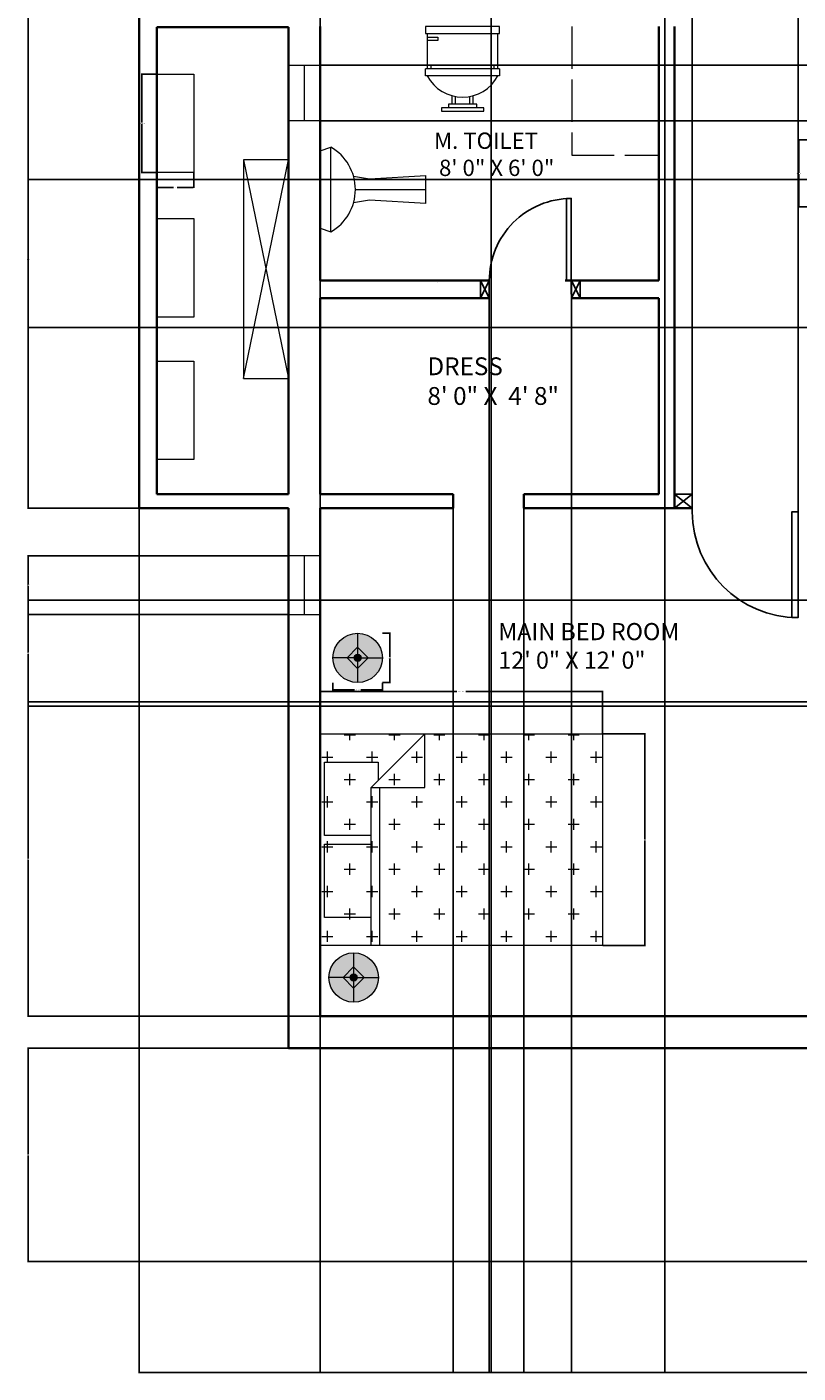
# Model space of a CAD drawing. Units: inches. Extents: x 2284228 to 3635239, y 3024422 to 8351872.
# Tile 1 of 7: x 3634669 to 3634888, y 8351218 to 8351600. Entities that reach past the tile are written whole.
import ezdxf

# ---------------------------------------------------------------- set-up
doc = ezdxf.new("R2010")
doc.units = ezdxf.units.IN
doc.linetypes.add('ACAD_ISO02W100', pattern=[15, 12, -3])
for name, color, linetype, lineweight in [('A-ANNO-DIMS', 2, 'Continuous', 18), ('A-AREA-IDEN', 7, 'Continuous', 18), ('A-DOOR', 4, 'Continuous', 25), ('A-EQPM', 8, 'Continuous', 18), ('A-FLOR-FIXT', 9, 'Continuous', 18), ('A-FLOR-FIXT-HIDN', 9, 'ACAD_ISO02W100', 18), ('A-FURN', 8, 'Continuous', 18), ('A-FURN-PATT', 9, 'Continuous', 13), ('A-GLAZ', 4, 'Continuous', 18), ('A-WALL', 7, 'Continuous', 35)]:
    doc.layers.add(name, color=color, linetype=linetype, lineweight=lineweight)
doc.styles.get("Standard").update_dxf_attribs({"font": 'arial.ttf'})
doc.dimstyles.get("Standard").update_dxf_attribs({"dimtxt": 0.18, "dimasz": 0.18, "dimexe": 0.18, "dimexo": 0.0625, "dimgap": 0.09, "dimtad": 0, "dimtih": 1, "dimtoh": 1, "dimdec": 4, "dimzin": 0, "dimdsep": 46, "dimtxsty": 'Standard', "dimcen": 0.09, "dimadec": 0, "dimazin": 0, "dimtfac": 1, "dimtdec": 4, "dimtofl": 0, "dimtmove": 0, "dimatfit": 3, "dimfxl": 1, "dimtolj": 1, "dimtzin": 0, "dimarcsym": 0})

# ---------------------------------------------------------------- blocks, each defined once
blk = doc.blocks.new('*U9')
for p, q in [((0, 0), (0, 5)), ((30, 0), (30, 5))]:
    blk.add_line(p, q)
blk.add_lwpolyline([(0, 0), (0, -30), (1.75, -30), (1.75, 0)], close=True)
blk.add_arc((0, 0), 30, 270, 0)
blk = doc.blocks.new('*U10')
for p, q in [((0, 0), (0, -5)), ((30, 0), (30, -5))]:
    blk.add_line(p, q)
blk.add_lwpolyline([(0, 0), (0, 30), (1.75, 30), (1.75, 0)], close=True)
blk.add_arc((0, 0), 30, 0, 90)
blk = doc.blocks.new('Bed - Queen')
for p, q in [((0, -80.00003), (0, 0)), ((0, 0), (59.99999, 0)), ((59.99999, 0), (59.99999, -80.00003)), ((7.99999, -1.2), (28.79998, -1.2)), ((7.99999, -14.4), (7.99999, -1.2)), ((28.79998, -1.2), (28.79998, -14.4)), ((31.19999, -1.2), (51.99999, -1.2)), ((31.19999, -14.4), (31.19999, -1.2)), ((51.99999, -1.2), (51.99999, -16.4)), ((0, -14.4), (44.8, -14.4)), ((59.99999, -29.6), (44.8, -14.4)), ((44.8, -14.4), (44.8, -29.6)), ((44.8, -16.8), (0, -16.8)), ((51.99999, -16.4), (46.79936, -16.4)), ((44.8, -29.6), (59.99999, -29.6)), ((59.99999, -80.00003), (0, -80.00003))]:
    blk.add_line(p, q)
blk = doc.blocks.new('Lamp - Table')
for p, q in [((0, 7), (0, 1)), ((-1, 0), (-7, 0)), ((0, 3), (-3, 0)), ((-3, 0), (0, -3)), ((3, 0), (0, 3)), ((0, -3), (3, 0)), ((1, 0), (7, 0)), ((0, -1), (0, -7))]:
    blk.add_line(p, q)
for radius in [7, 1]:
    blk.add_circle((0, 0), radius)
blk = doc.blocks.new('Toilet - Imperial')
for p, q in [((-10, 22), (-10, 12)), ((-10, 21), (-7, 21)), ((-7, 20), (-10, 20)), ((-7, 21), (-7, 20)), ((10, 12), (10, 22)), ((10.5, 12), (-10.5, 12)), ((-10.5, 10), (-10.5, 12)), ((9, 13), (-9, 13)), ((-9, 13), (-9, 12)), ((9, 12), (9, 13)), ((10.5, 12), (10.5, 10)), ((10.5, 10), (-10.5, 10)), ((-3, 4.4065), (-3, 2)), ((-2, 2), (-2, 4.1658)), ((2, 4.1658), (2, 2)), ((3, 2), (3, 4.4065)), ((4, 2), (-4, 2)), ((-4, 2), (-4, 1)), ((4, 1), (4, 2))]:
    blk.add_line(p, q)
for points in [[(10.5, 22), (10.5, 24), (-10.5, 24), (-10.5, 22)], [(6, 0), (6, 1), (-6, 1), (-6, 0)]]:
    blk.add_lwpolyline(points, close=True)
blk.add_arc((0, 15.3333), 11.3333, 208.0725, 331.9275)
blk = doc.blocks.new('Sink - Pedestal elevation')
for p, q in [((-11, 30), (-12, 27)), ((-12, 27), (12, 27)), ((-11, 30), (11, 30)), ((11, 30), (12, 27)), ((-3, 16), (-3.7523, 20.5139)), ((0, 20), (0, 0)), ((3.7527, 20.5157), (3, 16)), ((-4, 0), (-3, 16)), ((3, 16), (4, 0)), ((-4, 0), (4, 0))]:
    blk.add_line(p, q)
blk.add_arc((0, 33.7857), 13.7857, 209.4871, 330.5129)
blk = doc.blocks.new('SERVICE-LEDGE-MODULE')
blk.add_lwpolyline([(0, 10.53), (27.92, 10.53), (27.92, 0), (0, 0)], close=True)
blk = doc.blocks.new('*D22')
at = {"layer": 'A-ANNO-DIMS', "color": 0, "lineweight": -2, "transparency": 16777216}
for p, q in [((3634755.88, 8351414.07), (3634755.88, 8351411.85)), ((3634756.06, 8351412.03), (3634761.98, 8351412.03)), ((3634769.7, 8351412.03), (3634763.78, 8351412.03)), ((3634769.88, 8351414.07), (3634769.88, 8351411.85))]:
    blk.add_line(p, q, dxfattribs=at)
at = {"layer": 'A-ANNO-DIMS', "color": 0, "transparency": 16777216}
for points in [[(3634756.06, 8351412.06), (3634756.06, 8351412), (3634755.88, 8351412.03)], [(3634769.7, 8351412.06), (3634769.7, 8351412), (3634769.88, 8351412.03)]]:
    blk.add_solid(points, dxfattribs=at)
at = {"layer": 'Defpoints', "color": 0, "transparency": 16777216}
for p in [(3634755.88, 8351414.13), (3634769.88, 8351414.13), (3634769.88, 8351412.03)]:
    blk.add_point(p, dxfattribs=at)
at = {"layer": 'A-ANNO-DIMS', "color": 0, "transparency": 16777216, "insert": (3634762.88, 8351412.03), "char_height": 0.18, "attachment_point": 5}
blk.add_mtext('\\A1;LAMP 14 TYP.', dxfattribs=at)
blk = doc.blocks.new('*D23')
at = {"layer": 'A-ANNO-DIMS', "color": 0, "lineweight": -2, "transparency": 16777216}
for p, q in [((3634769.94, 8351428.13), (3634772.16, 8351428.13)), ((3634771.98, 8351427.95), (3634771.98, 8351421.32)), ((3634771.98, 8351414.31), (3634771.98, 8351420.95)), ((3634769.94, 8351414.13), (3634772.16, 8351414.13))]:
    blk.add_line(p, q, dxfattribs=at)
at = {"layer": 'A-ANNO-DIMS', "color": 0, "transparency": 16777216}
for points in [[(3634771.95, 8351427.95), (3634772.01, 8351427.95), (3634771.98, 8351428.13)], [(3634771.95, 8351414.31), (3634772.01, 8351414.31), (3634771.98, 8351414.13)]]:
    blk.add_solid(points, dxfattribs=at)
at = {"layer": 'Defpoints', "color": 0, "transparency": 16777216}
for p in [(3634769.88, 8351428.13), (3634771.98, 8351428.13), (3634769.88, 8351414.13)]:
    blk.add_point(p, dxfattribs=at)
at = {"layer": 'A-ANNO-DIMS', "color": 0, "transparency": 16777216, "insert": (3634771.98, 8351421.13), "char_height": 0.18, "attachment_point": 5}
blk.add_mtext('\\A1;14 TYP.', dxfattribs=at)
blk = doc.blocks.new('*D26')
at = {"layer": 'A-ANNO-DIMS', "color": 0, "lineweight": -2, "transparency": 16777216}
for p, q in [((3634890.78, 8351567.93), (3634887.82, 8351567.93)), ((3634888, 8351567.75), (3634888, 8351558.63)), ((3634888, 8351549.14), (3634888, 8351558.27)), ((3634890.79, 8351548.96), (3634887.82, 8351548.96))]:
    blk.add_line(p, q, dxfattribs=at)
at = {"layer": 'A-ANNO-DIMS', "color": 0, "transparency": 16777216}
for points in [[(3634888.03, 8351567.75), (3634887.97, 8351567.75), (3634888, 8351567.93)], [(3634888.03, 8351549.14), (3634887.97, 8351549.14), (3634888, 8351548.96)]]:
    blk.add_solid(points, dxfattribs=at)
at = {"layer": 'Defpoints', "color": 0, "transparency": 16777216}
for p in [(3634888, 8351567.93), (3634890.85, 8351567.93), (3634890.85, 8351548.96)]:
    blk.add_point(p, dxfattribs=at)
at = {"layer": 'A-ANNO-DIMS', "color": 0, "transparency": 16777216, "insert": (3634888, 8351558.45), "char_height": 0.18, "attachment_point": 5}
blk.add_mtext('\\A1;CHAIR 19 TYP.', dxfattribs=at)
blk = doc.blocks.new('*D28')
at = {"layer": 'A-ANNO-DIMS', "color": 0, "lineweight": -2, "transparency": 16777216}
for p, q in [((3634705.83, 8351586.6), (3634701.53, 8351586.6)), ((3634701.71, 8351586.42), (3634701.71, 8351572.82)), ((3634701.71, 8351558.86), (3634701.71, 8351572.46)), ((3634705.83, 8351558.68), (3634701.53, 8351558.68))]:
    blk.add_line(p, q, dxfattribs=at)
at = {"layer": 'A-ANNO-DIMS', "color": 0, "transparency": 16777216}
for points in [[(3634701.68, 8351586.42), (3634701.74, 8351586.42), (3634701.71, 8351586.6)], [(3634701.68, 8351558.86), (3634701.74, 8351558.86), (3634701.71, 8351558.68)]]:
    blk.add_solid(points, dxfattribs=at)
at = {"layer": 'Defpoints', "color": 0, "transparency": 16777216}
for p in [(3634701.71, 8351586.6), (3634705.9, 8351586.6), (3634705.9, 8351558.68)]:
    blk.add_point(p, dxfattribs=at)
at = {"layer": 'A-ANNO-DIMS', "color": 0, "transparency": 16777216, "insert": (3634701.71, 8351572.64), "char_height": 0.18, "attachment_point": 5}
blk.add_mtext('\\A1;LEDGE 28 TYP.', dxfattribs=at)
blk = doc.blocks.new('*D29')
at = {"layer": 'A-ANNO-DIMS', "color": 0, "lineweight": -2, "transparency": 16777216}
for p, q in [((3634705.9, 8351558.62), (3634705.9, 8351554.31)), ((3634716.43, 8351558.62), (3634716.43, 8351554.31)), ((3634706.08, 8351554.49), (3634710.64, 8351554.49)), ((3634716.25, 8351554.49), (3634711.68, 8351554.49))]:
    blk.add_line(p, q, dxfattribs=at)
at = {"layer": 'A-ANNO-DIMS', "color": 0, "transparency": 16777216}
for points in [[(3634706.08, 8351554.52), (3634706.08, 8351554.46), (3634705.9, 8351554.49)], [(3634716.25, 8351554.52), (3634716.25, 8351554.46), (3634716.43, 8351554.49)]]:
    blk.add_solid(points, dxfattribs=at)
at = {"layer": 'Defpoints', "color": 0, "transparency": 16777216}
for p in [(3634705.9, 8351558.68), (3634716.43, 8351558.68), (3634705.9, 8351554.49)]:
    blk.add_point(p, dxfattribs=at)
at = {"layer": 'A-ANNO-DIMS', "color": 0, "transparency": 16777216, "insert": (3634711.16, 8351554.49), "char_height": 0.18, "attachment_point": 5}
blk.add_mtext('\\A1;11 TYP.', dxfattribs=at)
blk = doc.blocks.new('*D30')
at = {"layer": 'A-ANNO-DIMS', "color": 0, "lineweight": -2, "transparency": 16777216}
for p, q in [((3634752.3, 8351399.63), (3634752.3, 8351411.75)), ((3634752.48, 8351411.57), (3634791, 8351411.57)), ((3634832.12, 8351411.57), (3634793.6, 8351411.57)), ((3634832.3, 8351399.63), (3634832.3, 8351411.75))]:
    blk.add_line(p, q, dxfattribs=at)
at = {"layer": 'A-ANNO-DIMS', "color": 0, "transparency": 16777216}
for points in [[(3634752.48, 8351411.6), (3634752.48, 8351411.54), (3634752.3, 8351411.57)], [(3634832.12, 8351411.6), (3634832.12, 8351411.54), (3634832.3, 8351411.57)]]:
    blk.add_solid(points, dxfattribs=at)
at = {"layer": 'Defpoints', "color": 0, "transparency": 16777216}
for p in [(3634752.3, 8351411.57), (3634752.3, 8351399.57), (3634832.3, 8351399.57)]:
    blk.add_point(p, dxfattribs=at)
at = {"layer": 'A-ANNO-DIMS', "color": 0, "transparency": 16777216, "insert": (3634792.3, 8351411.57), "char_height": 0.18, "attachment_point": 5}
blk.add_mtext('\\A1;QUEEN BED 80 TYP.', dxfattribs=at)
blk = doc.blocks.new('*D31')
at = {"layer": 'A-ANNO-DIMS', "color": 0, "lineweight": -2, "transparency": 16777216}
for p, q in [((3634832.36, 8351399.57), (3634844.48, 8351399.57)), ((3634844.3, 8351399.39), (3634844.3, 8351369.75)), ((3634844.3, 8351339.75), (3634844.3, 8351369.39)), ((3634832.36, 8351339.57), (3634844.48, 8351339.57))]:
    blk.add_line(p, q, dxfattribs=at)
at = {"layer": 'A-ANNO-DIMS', "color": 0, "transparency": 16777216}
for points in [[(3634844.27, 8351399.39), (3634844.33, 8351399.39), (3634844.3, 8351399.57)], [(3634844.27, 8351339.75), (3634844.33, 8351339.75), (3634844.3, 8351339.57)]]:
    blk.add_solid(points, dxfattribs=at)
at = {"layer": 'Defpoints', "color": 0, "transparency": 16777216}
for p in [(3634832.3, 8351399.57), (3634844.3, 8351399.57), (3634832.3, 8351339.57)]:
    blk.add_point(p, dxfattribs=at)
at = {"layer": 'A-ANNO-DIMS', "color": 0, "transparency": 16777216, "insert": (3634844.3, 8351369.57), "char_height": 0.18, "attachment_point": 5}
blk.add_mtext('\\A1;60 TYP.', dxfattribs=at)
blk = doc.blocks.new('*D40')
at = {"layer": 'A-ANNO-DIMS', "color": 0, "lineweight": -2, "transparency": 16777216}
for p, q in [((3634700.92, 8351463.5), (3634700.92, 8351218.43)), ((3635206.75, 8351310.5), (3635206.75, 8351218.43)), ((3634701.1, 8351218.61), (3634953.44, 8351218.61)), ((3635206.57, 8351218.61), (3634954.23, 8351218.61))]:
    blk.add_line(p, q, dxfattribs=at)
at = {"layer": 'A-ANNO-DIMS', "color": 0, "transparency": 16777216}
for points in [[(3634701.1, 8351218.64), (3634701.1, 8351218.58), (3634700.92, 8351218.61)], [(3635206.57, 8351218.64), (3635206.57, 8351218.58), (3635206.75, 8351218.61)]]:
    blk.add_solid(points, dxfattribs=at)
at = {"layer": 'Defpoints', "color": 0, "transparency": 16777216}
for p in [(3634700.92, 8351463.56), (3635206.75, 8351310.56), (3635206.75, 8351218.61)]:
    blk.add_point(p, dxfattribs=at)
at = {"layer": 'A-ANNO-DIMS', "color": 0, "transparency": 16777216, "insert": (3634953.83, 8351218.61), "char_height": 0.18, "attachment_point": 5}
blk.add_mtext('\\A1;505.8', dxfattribs=at)
blk = doc.blocks.new('*D46')
at = {"layer": 'A-ANNO-DIMS', "color": 0, "lineweight": -2, "transparency": 16777216}
for p, q in [((3634700.85, 8351604.4), (3634669.29, 8351604.4)), ((3634669.47, 8351604.22), (3634669.47, 8351534.17)), ((3634669.47, 8351463.74), (3634669.47, 8351533.8)), ((3634700.85, 8351463.56), (3634669.29, 8351463.56))]:
    blk.add_line(p, q, dxfattribs=at)
at = {"layer": 'A-ANNO-DIMS', "color": 0, "transparency": 16777216}
for points in [[(3634669.44, 8351604.22), (3634669.5, 8351604.22), (3634669.47, 8351604.4)], [(3634669.44, 8351463.74), (3634669.5, 8351463.74), (3634669.47, 8351463.56)]]:
    blk.add_solid(points, dxfattribs=at)
at = {"layer": 'Defpoints', "color": 0, "transparency": 16777216}
for p in [(3634669.47, 8351604.4), (3634700.92, 8351604.4), (3634700.92, 8351463.56)]:
    blk.add_point(p, dxfattribs=at)
at = {"layer": 'A-ANNO-DIMS', "color": 0, "transparency": 16777216, "insert": (3634669.47, 8351533.98), "char_height": 0.18, "attachment_point": 5}
blk.add_mtext('\\A1;140.84', dxfattribs=at)
blk = doc.blocks.new('*D48')
at = {"layer": 'A-ANNO-DIMS', "color": 0, "lineweight": -2, "transparency": 16777216}
for p, q in [((3634891.69, 8351310.56), (3634669.29, 8351310.56)), ((3634669.47, 8351310.38), (3634669.47, 8351280.49)), ((3634669.47, 8351250.24), (3634669.47, 8351280.13)), ((3634891.69, 8351250.06), (3634669.29, 8351250.06))]:
    blk.add_line(p, q, dxfattribs=at)
at = {"layer": 'A-ANNO-DIMS', "color": 0, "transparency": 16777216}
for points in [[(3634669.44, 8351310.38), (3634669.5, 8351310.38), (3634669.47, 8351310.56)], [(3634669.44, 8351250.24), (3634669.5, 8351250.24), (3634669.47, 8351250.06)]]:
    blk.add_solid(points, dxfattribs=at)
at = {"layer": 'Defpoints', "color": 0, "transparency": 16777216}
for p in [(3634669.47, 8351310.56), (3634891.75, 8351310.56), (3634891.75, 8351250.06)]:
    blk.add_point(p, dxfattribs=at)
at = {"layer": 'A-ANNO-DIMS', "color": 0, "transparency": 16777216, "insert": (3634669.47, 8351280.31), "char_height": 0.18, "attachment_point": 5}
blk.add_mtext('\\A1;60.5', dxfattribs=at)
blk = doc.blocks.new('*D50')
at = {"layer": 'A-ANNO-DIMS', "color": 0, "lineweight": -2, "transparency": 16777216}
for p, q in [((3634800.75, 8351748.5), (3634800.75, 8351218.43)), ((3634850, 8351748.5), (3634850, 8351218.43)), ((3634800.93, 8351218.61), (3634824.98, 8351218.61)), ((3634849.82, 8351218.61), (3634825.77, 8351218.61))]:
    blk.add_line(p, q, dxfattribs=at)
at = {"layer": 'A-ANNO-DIMS', "color": 0, "transparency": 16777216}
for points in [[(3634800.93, 8351218.64), (3634800.93, 8351218.58), (3634800.75, 8351218.61)], [(3634849.82, 8351218.64), (3634849.82, 8351218.58), (3634850, 8351218.61)]]:
    blk.add_solid(points, dxfattribs=at)
at = {"layer": 'Defpoints', "color": 0, "transparency": 16777216}
for p in [(3634800.75, 8351748.56), (3634850, 8351748.56), (3634850, 8351218.61)]:
    blk.add_point(p, dxfattribs=at)
at = {"layer": 'A-ANNO-DIMS', "color": 0, "transparency": 16777216, "insert": (3634825.37, 8351218.61), "char_height": 0.18, "attachment_point": 5}
blk.add_mtext('\\A1;49.25', dxfattribs=at)
blk = doc.blocks.new('*D51')
at = {"layer": 'A-ANNO-DIMS', "color": 0, "lineweight": -2, "transparency": 16777216}
for p, q in [((3634752.25, 8351748.5), (3634752.25, 8351218.43)), ((3634800.75, 8351748.5), (3634800.75, 8351218.43)), ((3634752.43, 8351218.61), (3634776.1, 8351218.61)), ((3634800.57, 8351218.61), (3634776.9, 8351218.61))]:
    blk.add_line(p, q, dxfattribs=at)
at = {"layer": 'A-ANNO-DIMS', "color": 0, "transparency": 16777216}
for points in [[(3634752.43, 8351218.64), (3634752.43, 8351218.58), (3634752.25, 8351218.61)], [(3634800.57, 8351218.64), (3634800.57, 8351218.58), (3634800.75, 8351218.61)]]:
    blk.add_solid(points, dxfattribs=at)
at = {"layer": 'Defpoints', "color": 0, "transparency": 16777216}
for p in [(3634752.25, 8351748.56), (3634800.75, 8351748.56), (3634800.75, 8351218.61)]:
    blk.add_point(p, dxfattribs=at)
at = {"layer": 'A-ANNO-DIMS', "color": 0, "transparency": 16777216, "insert": (3634776.5, 8351218.61), "char_height": 0.18, "attachment_point": 5}
blk.add_mtext('\\A1;48.49', dxfattribs=at)
blk = doc.blocks.new('*D60')
at = {"layer": 'A-ANNO-DIMS', "color": 0, "lineweight": -2, "transparency": 16777216}
for p, q in [((3635099.17, 8351408.67), (3634669.29, 8351408.67)), ((3634669.47, 8351408.49), (3634669.47, 8351364.3)), ((3634669.47, 8351319.74), (3634669.47, 8351363.93)), ((3635099.17, 8351319.56), (3634669.29, 8351319.56))]:
    blk.add_line(p, q, dxfattribs=at)
at = {"layer": 'A-ANNO-DIMS', "color": 0, "transparency": 16777216}
for points in [[(3634669.44, 8351408.49), (3634669.5, 8351408.49), (3634669.47, 8351408.67)], [(3634669.44, 8351319.74), (3634669.5, 8351319.74), (3634669.47, 8351319.56)]]:
    blk.add_solid(points, dxfattribs=at)
at = {"layer": 'Defpoints', "color": 0, "transparency": 16777216}
for p in [(3635099.24, 8351408.67), (3634669.47, 8351319.56), (3635099.24, 8351319.56)]:
    blk.add_point(p, dxfattribs=at)
at = {"layer": 'A-ANNO-DIMS', "color": 0, "transparency": 16777216, "insert": (3634669.47, 8351364.12), "char_height": 0.18, "attachment_point": 5}
blk.add_mtext('\\A1;89.1', dxfattribs=at)
blk = doc.blocks.new('*D69')
at = {"layer": 'A-ANNO-DIMS', "color": 0, "lineweight": -2, "transparency": 16777216}
for p, q in [((3634752.31, 8351589.14), (3635238.38, 8351589.14)), ((3635238.2, 8351588.96), (3635238.2, 8351581.41)), ((3635238.2, 8351573.51), (3635238.2, 8351581.05)), ((3634752.31, 8351573.33), (3635238.38, 8351573.33))]:
    blk.add_line(p, q, dxfattribs=at)
at = {"layer": 'A-ANNO-DIMS', "color": 0, "transparency": 16777216}
for points in [[(3635238.17, 8351588.96), (3635238.23, 8351588.96), (3635238.2, 8351589.14)], [(3635238.17, 8351573.51), (3635238.23, 8351573.51), (3635238.2, 8351573.33)]]:
    blk.add_solid(points, dxfattribs=at)
at = {"layer": 'Defpoints', "color": 0, "transparency": 16777216}
for p in [(3634752.25, 8351589.14), (3635238.2, 8351589.14), (3634752.25, 8351573.33)]:
    blk.add_point(p, dxfattribs=at)
at = {"layer": 'A-ANNO-DIMS', "color": 0, "transparency": 16777216, "insert": (3635238.2, 8351581.23), "char_height": 0.18, "attachment_point": 5}
blk.add_mtext('\\A1;15.813', dxfattribs=at)
blk = doc.blocks.new('*D70')
at = {"layer": 'A-ANNO-DIMS', "color": 0, "lineweight": -2, "transparency": 16777216}
for p, q in [((3634743.19, 8351450.1), (3634669.29, 8351450.1)), ((3634669.47, 8351449.92), (3634669.47, 8351441.94)), ((3634669.47, 8351433.6), (3634669.47, 8351441.58)), ((3634743.19, 8351433.42), (3634669.29, 8351433.42))]:
    blk.add_line(p, q, dxfattribs=at)
at = {"layer": 'A-ANNO-DIMS', "color": 0, "transparency": 16777216}
for points in [[(3634669.44, 8351449.92), (3634669.5, 8351449.92), (3634669.47, 8351450.1)], [(3634669.44, 8351433.6), (3634669.5, 8351433.6), (3634669.47, 8351433.42)]]:
    blk.add_solid(points, dxfattribs=at)
at = {"layer": 'Defpoints', "color": 0, "transparency": 16777216}
for p in [(3634669.47, 8351450.1), (3634743.25, 8351450.1), (3634743.25, 8351433.42)]:
    blk.add_point(p, dxfattribs=at)
at = {"layer": 'A-ANNO-DIMS', "color": 0, "transparency": 16777216, "insert": (3634669.47, 8351441.76), "char_height": 0.18, "attachment_point": 5}
blk.add_mtext('\\A1;16.683', dxfattribs=at)
blk = doc.blocks.new('*D75')
at = {"layer": 'A-ANNO-DIMS', "color": 0, "lineweight": -2, "transparency": 16777216}
for p, q in [((3634857.77, 8351463.63), (3634857.77, 8351830.64)), ((3634857.95, 8351830.46), (3634872.56, 8351830.46)), ((3634887.59, 8351830.46), (3634872.99, 8351830.46)), ((3634887.77, 8351463.63), (3634887.77, 8351830.64))]:
    blk.add_line(p, q, dxfattribs=at)
at = {"layer": 'A-ANNO-DIMS', "color": 0, "transparency": 16777216}
for points in [[(3634857.95, 8351830.49), (3634857.95, 8351830.43), (3634857.77, 8351830.46)], [(3634887.59, 8351830.49), (3634887.59, 8351830.43), (3634887.77, 8351830.46)]]:
    blk.add_solid(points, dxfattribs=at)
at = {"layer": 'Defpoints', "color": 0, "transparency": 16777216}
for p in [(3634887.77, 8351830.46), (3634857.77, 8351463.56), (3634887.77, 8351463.56)]:
    blk.add_point(p, dxfattribs=at)
at = {"layer": 'A-ANNO-DIMS', "color": 0, "transparency": 16777216, "insert": (3634872.77, 8351830.46), "char_height": 0.18, "attachment_point": 5}
blk.add_mtext('\\A1;30', dxfattribs=at)
blk = doc.blocks.new('*D76')
at = {"layer": 'A-ANNO-DIMS', "color": 0, "lineweight": -2, "transparency": 16777216}
for p, q in [((3634789.93, 8351463.5), (3634789.93, 8351218.43)), ((3634810.01, 8351463.5), (3634810.01, 8351218.43)), ((3634790.11, 8351218.61), (3634799.51, 8351218.61)), ((3634809.83, 8351218.61), (3634800.44, 8351218.61))]:
    blk.add_line(p, q, dxfattribs=at)
at = {"layer": 'A-ANNO-DIMS', "color": 0, "transparency": 16777216}
for points in [[(3634790.11, 8351218.64), (3634790.11, 8351218.58), (3634789.93, 8351218.61)], [(3634809.83, 8351218.64), (3634809.83, 8351218.58), (3634810.01, 8351218.61)]]:
    blk.add_solid(points, dxfattribs=at)
at = {"layer": 'Defpoints', "color": 0, "transparency": 16777216}
for p in [(3634789.93, 8351463.56), (3634810.01, 8351463.56), (3634810.01, 8351218.61)]:
    blk.add_point(p, dxfattribs=at)
at = {"layer": 'A-ANNO-DIMS', "color": 0, "transparency": 16777216, "insert": (3634799.97, 8351218.61), "char_height": 0.18, "attachment_point": 5}
blk.add_mtext('\\A1;20.078', dxfattribs=at)
blk = doc.blocks.new('*D77')
at = {"layer": 'A-ANNO-DIMS', "color": 0, "lineweight": -2, "transparency": 16777216}
for p, q in [((3634800.2, 8351523), (3634800.2, 8351218.43)), ((3634823.48, 8351523), (3634823.48, 8351218.43)), ((3634800.38, 8351218.61), (3634811.38, 8351218.61)), ((3634823.3, 8351218.61), (3634812.31, 8351218.61))]:
    blk.add_line(p, q, dxfattribs=at)
at = {"layer": 'A-ANNO-DIMS', "color": 0, "transparency": 16777216}
for points in [[(3634800.38, 8351218.64), (3634800.38, 8351218.58), (3634800.2, 8351218.61)], [(3634823.3, 8351218.64), (3634823.3, 8351218.58), (3634823.48, 8351218.61)]]:
    blk.add_solid(points, dxfattribs=at)
at = {"layer": 'Defpoints', "color": 0, "transparency": 16777216}
for p in [(3634800.2, 8351523.07), (3634823.48, 8351523.06), (3634823.48, 8351218.61)]:
    blk.add_point(p, dxfattribs=at)
at = {"layer": 'A-ANNO-DIMS', "color": 0, "transparency": 16777216, "insert": (3634811.84, 8351218.61), "char_height": 0.18, "attachment_point": 5}
blk.add_mtext('\\A1;23.277', dxfattribs=at)
blk = doc.blocks.new('*D79')
at = {"layer": 'A-ANNO-DIMS', "color": 0, "lineweight": -2, "transparency": 16777216}
for p, q in [((3635095.53, 8351556.72), (3634669.29, 8351556.72)), ((3634669.47, 8351556.54), (3634669.47, 8351535.9)), ((3634669.47, 8351514.9), (3634669.47, 8351535.54)), ((3635095.53, 8351514.72), (3634669.29, 8351514.72))]:
    blk.add_line(p, q, dxfattribs=at)
at = {"layer": 'A-ANNO-DIMS', "color": 0, "transparency": 16777216}
for points in [[(3634669.44, 8351556.54), (3634669.5, 8351556.54), (3634669.47, 8351556.72)], [(3634669.44, 8351514.9), (3634669.5, 8351514.9), (3634669.47, 8351514.72)]]:
    blk.add_solid(points, dxfattribs=at)
at = {"layer": 'Defpoints', "color": 0, "transparency": 16777216}
for p in [(3634669.47, 8351556.72), (3635095.59, 8351556.72), (3635095.59, 8351514.72)]:
    blk.add_point(p, dxfattribs=at)
at = {"layer": 'A-ANNO-DIMS', "color": 0, "transparency": 16777216, "insert": (3634669.47, 8351535.72), "char_height": 0.18, "attachment_point": 5}
blk.add_mtext('\\A1;42', dxfattribs=at)
blk = doc.blocks.new('*D81')
at = {"layer": 'A-ANNO-DIMS', "color": 0, "lineweight": -2, "transparency": 16777216}
for p, q in [((3634948.68, 8351437.49), (3634669.29, 8351437.49)), ((3634669.47, 8351437.31), (3634669.47, 8351422.68)), ((3634669.47, 8351407.67), (3634669.47, 8351422.31)), ((3634948.68, 8351407.49), (3634669.29, 8351407.49))]:
    blk.add_line(p, q, dxfattribs=at)
at = {"layer": 'A-ANNO-DIMS', "color": 0, "transparency": 16777216}
for points in [[(3634669.44, 8351437.31), (3634669.5, 8351437.31), (3634669.47, 8351437.49)], [(3634669.44, 8351407.67), (3634669.5, 8351407.67), (3634669.47, 8351407.49)]]:
    blk.add_solid(points, dxfattribs=at)
at = {"layer": 'Defpoints', "color": 0, "transparency": 16777216}
for p in [(3634669.47, 8351437.49), (3634948.75, 8351437.49), (3634948.75, 8351407.49)]:
    blk.add_point(p, dxfattribs=at)
at = {"layer": 'A-ANNO-DIMS', "color": 0, "transparency": 16777216, "insert": (3634669.47, 8351422.49), "char_height": 0.18, "attachment_point": 5}
blk.add_mtext('\\A1;30', dxfattribs=at)

msp = doc.modelspace()

# ---------------------------------------------------------------- hatches: boundary and pattern name
at = {"layer": 'A-FURN-PATT'}
h = msp.add_hatch(color=256, dxfattribs=at)
h.dxf.hatch_style = 1
h.paths.add_polyline_path([(3634761.747, 8351337.5419), (3634761.747, 8351333.5419), (3634764.747, 8351330.5419), (3634768.747, 8351330.5419, 0.41421356)])
h.paths.add_polyline_path([(3634761.747, 8351337.5419, 0.41421356), (3634754.747, 8351330.5419), (3634758.747, 8351330.5419), (3634761.747, 8351333.5419)])
h.paths.add_polyline_path([(3634758.747, 8351330.5419), (3634754.747, 8351330.5419, 0.41421356), (3634761.747, 8351323.5419), (3634761.747, 8351327.5419)])
h.paths.add_polyline_path([(3634768.747, 8351330.5419), (3634764.747, 8351330.5419), (3634761.747, 8351327.5419), (3634761.747, 8351323.5419, 0.41421356)])
h.paths.add_polyline_path([(3634762.881, 8351428.1349, 0.41421356), (3634755.881, 8351421.1349), (3634759.881, 8351421.1349), (3634762.881, 8351424.1349)])
h.paths.add_polyline_path([(3634762.881, 8351428.1349), (3634762.881, 8351424.1349), (3634765.881, 8351421.1349), (3634769.881, 8351421.1349, 0.41421356)])
h.paths.add_polyline_path([(3634769.881, 8351421.1349), (3634765.881, 8351421.1349), (3634762.881, 8351418.1349), (3634762.881, 8351414.1349, 0.41421356)])
h.paths.add_polyline_path([(3634762.881, 8351418.1349), (3634759.881, 8351421.1349), (3634755.881, 8351421.1349, 0.41421356), (3634762.881, 8351414.1349)])
h = msp.add_hatch(color=256, dxfattribs=at)
h.dxf.hatch_style = 1
h.paths.add_polyline_path([(3634762.881, 8351424.1349), (3634759.881, 8351421.1349), (3634761.881, 8351421.1349, -0.41421356), (3634762.881, 8351422.1349)])
h.paths.add_polyline_path([(3634762.881, 8351424.1349), (3634762.881, 8351422.1349, -0.41421356), (3634763.881, 8351421.1349), (3634765.881, 8351421.1349)])
h.paths.add_polyline_path([(3634765.881, 8351421.1349), (3634763.881, 8351421.1349, -0.41421356), (3634762.881, 8351420.1349), (3634762.881, 8351418.1349)])
h.paths.add_polyline_path([(3634762.881, 8351420.1349, -0.41421356), (3634761.881, 8351421.1349), (3634759.881, 8351421.1349), (3634762.881, 8351418.1349)])
h.paths.add_polyline_path([(3634761.747, 8351333.5419), (3634758.747, 8351330.5419), (3634760.747, 8351330.5419, -0.41421356), (3634761.747, 8351331.5419)])
h.paths.add_polyline_path([(3634761.747, 8351333.5419), (3634761.747, 8351331.5419, -0.41421356), (3634762.747, 8351330.5419), (3634764.747, 8351330.5419)])
h.paths.add_polyline_path([(3634764.747, 8351330.5419), (3634762.747, 8351330.5419, -0.41421356), (3634761.747, 8351329.5419), (3634761.747, 8351327.5419)])
h.paths.add_polyline_path([(3634761.747, 8351329.5419, -0.41421356), (3634760.747, 8351330.5419), (3634758.747, 8351330.5419), (3634761.747, 8351327.5419)])
h = msp.add_hatch(color=256, dxfattribs=at)
h.dxf.hatch_style = 1
h.paths.add_polyline_path([(3634763.881, 8351421.1349, 1), (3634761.881, 8351421.1349, 1)])
h = msp.add_hatch(dxfattribs=at)
h.set_pattern_fill('CROSS', color=256)
h.paths.add_polyline_path([(3634832.2997, 8351399.5692), (3634781.8997, 8351399.5692), (3634781.8997, 8351384.3692), (3634769.0997, 8351384.3692), (3634769.0997, 8351339.5692), (3634832.2997, 8351339.5692)])
h.paths.add_polyline_path([(3634781.8997, 8351399.5692), (3634752.2997, 8351399.5692), (3634752.2997, 8351339.5692), (3634766.6997, 8351339.5692), (3634766.6997, 8351347.5692), (3634753.4997, 8351347.5692), (3634753.4997, 8351368.3692), (3634766.6997, 8351368.3692), (3634766.6997, 8351370.7692), (3634753.4997, 8351370.7692), (3634753.4997, 8351391.5692), (3634768.6997, 8351391.5692), (3634768.6997, 8351386.3692)], flags=17)
h.paths.add_polyline_path([(3634781.8997, 8351399.5692), (3634766.6997, 8351384.3692), (3634781.8997, 8351384.3692)], flags=0)
h.paths.add_polyline_path([(3634768.6997, 8351391.5692), (3634753.4997, 8351391.5692), (3634753.4997, 8351370.7692), (3634766.6997, 8351370.7692), (3634766.6997, 8351384.3692), (3634768.6997, 8351386.3692)], flags=0)
h.paths.add_polyline_path([(3634766.6997, 8351368.3692), (3634753.4997, 8351368.3692), (3634753.4997, 8351347.5692), (3634766.6997, 8351347.5692)], flags=0)
h.paths.add_polyline_path([(3634766.6997, 8351347.5692), (3634753.4997, 8351347.5692), (3634753.4997, 8351368.3692), (3634766.6997, 8351368.3692), (3634766.6997, 8351370.7692), (3634753.4997, 8351370.7692), (3634753.4997, 8351391.5692), (3634768.6997, 8351391.5692), (3634768.6997, 8351386.3692), (3634781.8997, 8351399.5692), (3634752.2997, 8351399.5692), (3634752.2997, 8351339.5692), (3634766.6997, 8351339.5692)], flags=17)
h.paths.add_polyline_path([(3634766.6997, 8351384.3692), (3634768.6997, 8351386.3692), (3634768.6997, 8351391.5692), (3634753.4997, 8351391.5692), (3634753.4997, 8351370.7692), (3634766.6997, 8351370.7692)], flags=0)
h.paths.add_polyline_path([(3634781.8997, 8351399.5692), (3634768.6997, 8351386.3692), (3634766.6997, 8351384.3692), (3634781.8997, 8351384.3692)], flags=0)
h.paths.add_polyline_path([(3634768.6997, 8351386.3692), (3634768.6997, 8351391.5692), (3634753.4997, 8351391.5692), (3634753.4997, 8351370.7692), (3634766.6997, 8351370.7692), (3634766.6997, 8351384.3692)], flags=0)
h = msp.add_hatch(dxfattribs=at)
h.set_pattern_fill('CROSS', color=256)
h.paths.add_polyline_path([(3634781.8997, 8351399.5692), (3634766.6997, 8351384.3692), (3634781.8997, 8351384.3692)], flags=0)
h.paths.add_polyline_path([(3634781.8997, 8351399.5692), (3634752.2997, 8351399.5692), (3634752.2997, 8351339.5692), (3634766.6997, 8351339.5692), (3634766.6997, 8351347.5692), (3634753.4997, 8351347.5692), (3634753.4997, 8351368.3692), (3634766.6997, 8351368.3692), (3634766.6997, 8351370.7692), (3634753.4997, 8351370.7692), (3634753.4997, 8351391.5692), (3634768.6997, 8351391.5692), (3634768.6997, 8351386.3692)], flags=17)
h.paths.add_polyline_path([(3634766.6997, 8351384.3692), (3634768.6997, 8351386.3692), (3634768.6997, 8351391.5692), (3634753.4997, 8351391.5692), (3634753.4997, 8351370.7692), (3634766.6997, 8351370.7692)], flags=0)
h.paths.add_polyline_path([(3634769.0997, 8351384.3692), (3634766.6997, 8351384.3692), (3634766.6997, 8351339.5692), (3634769.0997, 8351339.5692)], flags=0)
h.paths.add_polyline_path([(3634766.6997, 8351368.3692), (3634753.4997, 8351368.3692), (3634753.4997, 8351347.5692), (3634766.6997, 8351347.5692)], flags=0)
h.paths.add_polyline_path([(3634766.6997, 8351347.5692), (3634753.4997, 8351347.5692), (3634753.4997, 8351368.3692), (3634766.6997, 8351368.3692), (3634766.6997, 8351370.7692), (3634753.4997, 8351370.7692), (3634753.4997, 8351391.5692), (3634768.6997, 8351391.5692), (3634768.6997, 8351386.3692), (3634781.8997, 8351399.5692), (3634752.2997, 8351399.5692), (3634752.2997, 8351339.5692), (3634766.6997, 8351339.5692)], flags=17)
h.paths.add_polyline_path([(3634781.8997, 8351399.5692), (3634768.6997, 8351386.3692), (3634766.6997, 8351384.3692), (3634769.0997, 8351384.3692), (3634781.8997, 8351384.3692)], flags=0)
h = msp.add_hatch(dxfattribs=at)
h.set_pattern_fill('CROSS', color=256)
h.paths.add_polyline_path([(3634781.8997, 8351399.5692), (3634766.6997, 8351384.3692), (3634781.8997, 8351384.3692)], flags=17)
h.paths.add_polyline_path([(3634766.6997, 8351384.3692), (3634768.6997, 8351386.3692), (3634768.6997, 8351391.5692), (3634753.4997, 8351391.5692), (3634753.4997, 8351370.7692), (3634766.6997, 8351370.7692)], flags=17)
h.paths.add_polyline_path([(3634769.0997, 8351384.3692), (3634766.6997, 8351384.3692), (3634766.6997, 8351339.5692), (3634769.0997, 8351339.5692)], flags=17)
h.paths.add_polyline_path([(3634766.6997, 8351368.3692), (3634753.4997, 8351368.3692), (3634753.4997, 8351347.5692), (3634766.6997, 8351347.5692)], flags=17)
h.paths.add_polyline_path([(3634766.6997, 8351347.5692), (3634753.4997, 8351347.5692), (3634753.4997, 8351368.3692), (3634766.6997, 8351368.3692), (3634766.6997, 8351370.7692), (3634753.4997, 8351370.7692), (3634753.4997, 8351391.5692), (3634768.6997, 8351391.5692), (3634768.6997, 8351386.3692), (3634781.8997, 8351399.5692), (3634752.2997, 8351399.5692), (3634752.2997, 8351339.5692), (3634766.6997, 8351339.5692)])
h = msp.add_hatch(color=256, dxfattribs=at)
h.dxf.hatch_style = 1
h.paths.add_polyline_path([(3634760.747, 8351330.5419, 1), (3634762.747, 8351330.5419, 1)])

# ---------------------------------------------------------------- linework, layer by layer
at = {"layer": 'A-DOOR'}
for p, q in [((3634797.6819, 8351528.0663), (3634797.6819, 8351523.0663)), ((3634797.6819, 8351528.0663), (3634800.2032, 8351523.0663)), ((3634797.6819, 8351523.0663), (3634800.2032, 8351528.0663)), ((3634800.2032, 8351528.0663), (3634800.2032, 8351523.0663)), ((3634823.48, 8351528.0627), (3634823.48, 8351523.0627)), ((3634823.48, 8351528.0627), (3634826.0013, 8351523.0627)), ((3634823.48, 8351523.0627), (3634826.0013, 8351528.0627)), ((3634826.0013, 8351528.0627), (3634826.0013, 8351523.0627)), ((3634852.7525, 8351467.5627), (3634857.7742, 8351463.5627)), ((3634852.7525, 8351467.5627), (3634857.7742, 8351467.5627)), ((3634852.7525, 8351463.5627), (3634857.7742, 8351467.5472))]:
    msp.add_line(p, q, dxfattribs=at)
at = {"layer": 'A-EQPM'}
for p, q in [((3634730.539, 8351562.2635), (3634743.2525, 8351500.3574)), ((3634730.539, 8351500.3574), (3634743.2525, 8351562.2635))]:
    msp.add_line(p, q, dxfattribs=at)
msp.add_lwpolyline([(3634743.2525, 8351562.2635), (3634730.539, 8351562.2635), (3634730.539, 8351500.3574), (3634743.2525, 8351500.3574)], close=True, dxfattribs=at)
at = {"layer": 'A-FLOR-FIXT-HIDN'}
for p, q in [((3634823.6028, 8351600.0627), (3634823.6028, 8351563.6068)), ((3634823.6028, 8351563.6068), (3634848.1605, 8351563.6068))]:
    msp.add_line(p, q, dxfattribs=at)
at = {"layer": 'A-GLAZ'}
for p, q in [((3634743.2525, 8351589.1383), (3634752.2525, 8351589.1383)), ((3634747.7525, 8351589.1383), (3634747.7525, 8351573.3256)), ((3634752.2525, 8351589.1383), (3634752.2525, 8351573.3256)), ((3634752.2525, 8351573.3256), (3634743.2525, 8351573.3256)), ((3634743.2525, 8351450.1023), (3634752.2525, 8351450.1023)), ((3634747.7525, 8351450.1023), (3634747.7525, 8351433.4197)), ((3634743.2525, 8351433.4197), (3634752.2525, 8351433.4197))]:
    msp.add_line(p, q, dxfattribs=at)
at = {"layer": 'A-WALL'}
for p, q in [((3634700.915, 8351463.5627), (3634700.915, 8351604.405)), ((3634705.8958, 8351467.5627), (3634705.8958, 8351599.905)), ((3634743.2525, 8351599.905), (3634705.8958, 8351599.905)), ((3634743.2525, 8351467.5627), (3634743.2525, 8351599.905)), ((3634752.2525, 8351528.0627), (3634752.2525, 8351600.0627)), ((3634848.2525, 8351528.0627), (3634848.2525, 8351600.0627)), ((3634848.2525, 8351528.0627), (3634848.2525, 8351600.0627)), ((3634852.7525, 8351463.5627), (3634852.7525, 8351600.0627)), ((3634752.2525, 8351528.0627), (3634800.202, 8351528.0684)), ((3634785.4995, 8351527.5722), (3634785.5039, 8351527.581)), ((3634785.4995, 8351527.5722), (3634785.5051, 8351527.5722)), ((3634821.7172, 8351528.0627), (3634848.2525, 8351528.0627)), ((3634752.2525, 8351523.0627), (3634800.202, 8351523.0627)), ((3634752.2525, 8351467.5627), (3634752.2525, 8351523.0627)), ((3634823.4672, 8351523.0627), (3634848.2525, 8351523.0627)), ((3634848.2525, 8351467.5627), (3634848.2525, 8351523.0627)), ((3634848.2525, 8351467.5627), (3634848.2525, 8351523.0627)), ((3634705.8958, 8351467.5627), (3634743.2525, 8351467.5627)), ((3634752.2525, 8351467.5627), (3634789.9315, 8351467.5627)), ((3634789.9315, 8351467.5627), (3634789.9315, 8351463.5627)), ((3634810.0095, 8351467.5627), (3634810.0095, 8351463.5627)), ((3634810.0095, 8351467.5627), (3634848.2525, 8351467.5627)), ((3634700.915, 8351463.5627), (3634743.2525, 8351463.5627)), ((3634743.2525, 8351310.5627), (3634743.2525, 8351463.5627)), ((3634752.2525, 8351319.5627), (3634752.2525, 8351463.5627)), ((3634752.2525, 8351463.5627), (3634789.9315, 8351463.5627)), ((3634810.0095, 8351463.5627), (3634857.7742, 8351463.5627)), ((3634752.2525, 8351319.5627), (3634896.2525, 8351319.5627)), ((3634752.2525, 8351319.5627), (3634896.2525, 8351319.5627)), ((3634743.2525, 8351310.5627), (3634891.7525, 8351310.5627))]:
    msp.add_line(p, q, dxfattribs=at)
msp.add_lwpolyline([(3634705.8958, 8351467.5627), (3634705.8958, 8351493.6787)], dxfattribs=at)

# ---------------------------------------------------------------- block references
at = {"layer": 'A-DOOR', "xscale": 0.7755041374691896, "yscale": 0.7755041374691896, "zscale": 0.7755041374691896, "rotation": 180}
msp.add_blockref('*U9', (3634823.4672, 8351528.0684), dxfattribs=at)
at = {"layer": 'A-DOOR', "rotation": 180}
msp.add_blockref('*U10', (3634887.7742, 8351462.5472), dxfattribs=at)
at = {"layer": 'A-EQPM'}
for p, rotation in [((3634716.4298, 8351558.6786), 90.00000000418257), ((3634716.4298, 8351517.6975), 90.00000000313058), ((3634716.4298, 8351477.3304), 90.00000000313058)]:
    msp.add_blockref('SERVICE-LEDGE-MODULE', p, dxfattribs=dict(at, rotation=rotation))
at = {"layer": 'A-FLOR-FIXT'}
msp.add_blockref('Toilet - Imperial', (3634792.6326, 8351576.0627), dxfattribs=at)
at = {"layer": 'A-FLOR-FIXT', "rotation": 89.99999999999999}
msp.add_blockref('Sink - Pedestal elevation', (3634782.249, 8351553.8736), dxfattribs=at)
at = {"layer": 'A-FURN'}
for p in [(3634762.881, 8351421.1349), (3634761.747, 8351330.5419)]:
    msp.add_blockref('Lamp - Table', p, dxfattribs=at)
at = {"layer": 'A-FURN', "rotation": 90}
msp.add_blockref('Bed - Queen', (3634752.2997, 8351339.5692), dxfattribs=at)

# ---------------------------------------------------------------- texts
at = {"layer": 'A-AREA-IDEN', "attachment_point": 1}
for s, width, gutter_width, insert, char_height in [('   M. TOILET\\P    8\' 0" X 6\' 0"', 87.840894, 23.0839, (3634780.3133, 8351570.0172), 4.616781), ('     DRESS\\P     8\' 0" X  4\' 8"', 162.78312, 25.2346, (3634774.9551, 8351506.2973), 5.046912), ('     MAIN BED ROOM\\P     12\' 0" X 12\' 0"', 163.631376, 24.2751, (3634795.345, 8351431.0065), 4.855017)]:
    msp.add_mtext_dynamic_manual_height_columns(s, width=width, gutter_width=gutter_width, heights=[0], dxfattribs=dict(at, insert=insert, char_height=char_height))

# ---------------------------------------------------------------- dimensions: what is measured, and where the dimension line sits
at = {"layer": 'A-ANNO-DIMS'}
for base, p1, p2, override, picture, middle in [((3634887.7742, 8351830.4618), (3634857.7742, 8351463.5627), (3634887.7742, 8351463.5627), {"dimdec": 0, "dimlfac": 1, "dimrnd": 0, "dimzin": 0, "dimdsep": 46, "dimlunit": 2}, '*D75', (3634872.7742, 8351830.4618)), ((3634800.7459, 8351218.6127), (3634752.2525, 8351748.5627), (3634800.7459, 8351748.5627), {"dimdec": 2, "dimlfac": 1, "dimrnd": 0, "dimzin": 0, "dimdsep": 46, "dimlunit": 2}, '*D51', (3634776.4992, 8351218.6127)), ((3634850.0004, 8351218.6127), (3634800.7459, 8351748.5627), (3634850.0004, 8351748.5627), {"dimdec": 2, "dimlfac": 1, "dimrnd": 0, "dimzin": 0, "dimdsep": 46, "dimlunit": 2}, '*D50', (3634825.3732, 8351218.6127)), ((3634823.48, 8351218.6127), (3634800.2032, 8351523.0663), (3634823.48, 8351523.0627), {"dimdec": 3, "dimlfac": 1, "dimrnd": 0, "dimzin": 0, "dimdsep": 46, "dimlunit": 2}, '*D77', (3634811.8416, 8351218.6127)), ((3635206.7525, 8351218.6127), (3634700.915, 8351463.5627), (3635206.7525, 8351310.5627), {"dimdec": 1, "dimlfac": 1, "dimrnd": 0, "dimzin": 0, "dimdsep": 46, "dimlunit": 2}, '*D40', (3634953.8337, 8351218.6127)), ((3634810.0095, 8351218.6127), (3634789.9315, 8351463.5627), (3634810.0095, 8351463.5627), {"dimdec": 3, "dimlfac": 1, "dimrnd": 0, "dimzin": 0, "dimdsep": 46, "dimlunit": 2}, '*D76', (3634799.9705, 8351218.6127))]:
    dim = msp.add_linear_dim(base=base, p1=p1, p2=p2, dimstyle='Standard', override=override, dxfattribs=at)
    dim.commit()
    dim.dimension.update_dxf_attribs({"geometry": picture, "text_midpoint": middle})
for base, p1, p2, override, picture, middle in [((3634669.465, 8351604.405), (3634700.915, 8351463.5627), (3634700.915, 8351604.405), {"dimdec": 2, "dimlfac": 1, "dimrnd": 0, "dimzin": 0, "dimdsep": 46, "dimlunit": 2}, '*D46', (3634669.465, 8351533.9838)), ((3635238.2025, 8351589.1383), (3634752.2525, 8351573.3256), (3634752.2525, 8351589.1383), {"dimdec": 3, "dimlfac": 1, "dimrnd": 0, "dimzin": 0, "dimdsep": 46, "dimlunit": 2}, '*D69', (3635238.2025, 8351581.232)), ((3634669.465, 8351556.7209), (3635095.5898, 8351514.7209), (3635095.5898, 8351556.7209), {"dimdec": 0, "dimlfac": 1, "dimrnd": 0, "dimzin": 0, "dimdsep": 46, "dimlunit": 2}, '*D79', (3634669.465, 8351535.7209)), ((3634669.465, 8351450.1023), (3634743.2525, 8351433.4197), (3634743.2525, 8351450.1023), {"dimdec": 3, "dimlfac": 1, "dimrnd": 0, "dimzin": 0, "dimdsep": 46, "dimlunit": 2}, '*D70', (3634669.465, 8351441.761)), ((3634669.465, 8351437.4931), (3634948.7462, 8351407.4931), (3634948.7462, 8351437.4931), {"dimdec": 0, "dimlfac": 1, "dimrnd": 0, "dimzin": 0, "dimdsep": 46, "dimlunit": 2}, '*D81', (3634669.465, 8351422.4931)), ((3634669.465, 8351319.5627), (3635099.2364, 8351408.6677), (3635099.2364, 8351319.5627), {"dimdec": 1, "dimlfac": 1, "dimrnd": 0, "dimzin": 0, "dimdsep": 46, "dimlunit": 2}, '*D60', (3634669.465, 8351364.1152)), ((3634669.465, 8351310.5627), (3634891.7525, 8351250.0627), (3634891.7525, 8351310.5627), {"dimdec": 1, "dimlfac": 1, "dimrnd": 0, "dimzin": 0, "dimdsep": 46, "dimlunit": 2}, '*D48', (3634669.465, 8351280.3127))]:
    dim = msp.add_linear_dim(base=base, p1=p1, p2=p2, angle=90, dimstyle='Standard', override=override, dxfattribs=at)
    dim.commit()
    dim.dimension.update_dxf_attribs({"geometry": picture, "text_midpoint": middle})
for base, p1, p2, angle, text, picture, middle in [((3634701.7077, 8351586.5988), (3634705.8958, 8351558.6782), (3634705.8958, 8351586.5988), 90, 'LEDGE <> TYP.', '*D28', (3634701.7077, 8351572.6385)), ((3634888.0021, 8351567.934), (3634890.8494, 8351548.9648), (3634890.8475, 8351567.9343), 90.00585, 'CHAIR <> TYP.', '*D26', (3634888.003, 8351558.4492)), ((3634705.8958, 8351554.4901), (3634716.4297, 8351558.6782), (3634705.8958, 8351558.6782), 180, '<> TYP.', '*D29', (3634711.1627, 8351554.4901)), ((3634771.981, 8351428.1349), (3634769.881, 8351414.1349), (3634769.881, 8351428.1349), 90, '<> TYP.', '*D23', (3634771.981, 8351421.1349)), ((3634752.2997, 8351411.5692), (3634832.2997, 8351399.5692), (3634752.2997, 8351399.5692), 180, 'QUEEN BED <> TYP.', '*D30', (3634792.2997, 8351411.5692)), ((3634844.2997, 8351399.5692), (3634832.2997, 8351339.5692), (3634832.2997, 8351399.5692), 90, '<> TYP.', '*D31', (3634844.2997, 8351369.5692))]:
    dim = msp.add_linear_dim(base=base, p1=p1, p2=p2, angle=angle, text=text, dimstyle='Standard', override={"dimdec": 0, "dimlfac": 1, "dimrnd": 0, "dimzin": 0, "dimdsep": 46, "dimlunit": 2}, dxfattribs=at)
    dim.commit()
    dim.dimension.update_dxf_attribs({"geometry": picture, "text_midpoint": middle})
dim = msp.add_linear_dim(base=(3634769.881, 8351412.0349), p1=(3634755.881, 8351414.1349), p2=(3634769.881, 8351414.1349), text='LAMP <> TYP.', dimstyle='Standard', override={"dimdec": 0, "dimlfac": 1, "dimrnd": 0, "dimzin": 0, "dimdsep": 46, "dimlunit": 2}, dxfattribs=at)
dim.commit()
dim.dimension.update_dxf_attribs({"geometry": '*D22', "text_midpoint": (3634762.881, 8351412.0349)})

doc.saveas('drawing.dxf')
